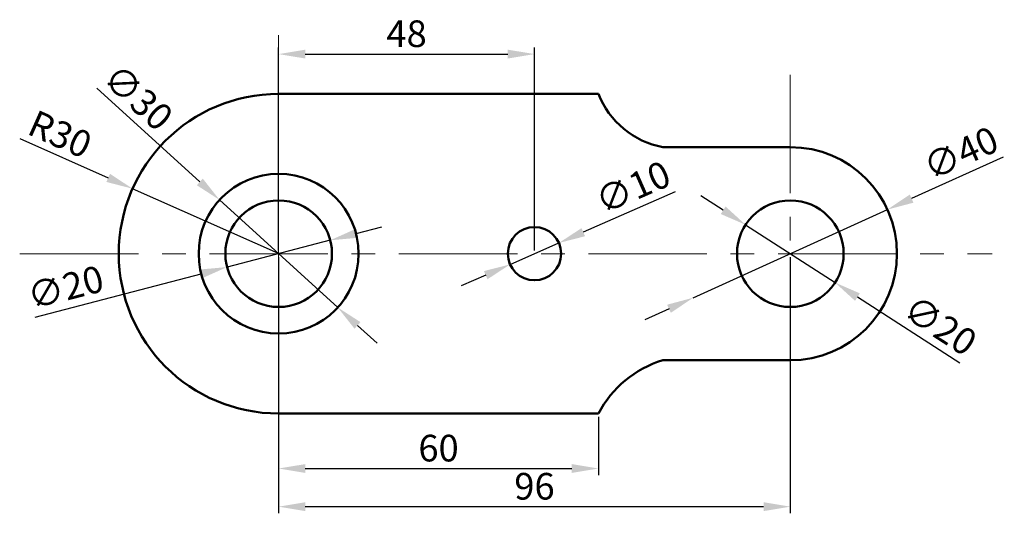
# Model space of a CAD drawing. Units: millimetres. Extents: x 1950 to 2135, y 1566 to 1659.
import ezdxf

# ---------------------------------------------------------------- set-up
doc = ezdxf.new("R2010")
doc.units = ezdxf.units.MM
doc.linetypes.add('CENTER', pattern=[50.8, 31.75, -6.35, 6.35, -6.35])
for name, color, linetype, lineweight in [('M-CNTR', 4, 'CENTER', 18), ('M-DIMS', 2, 'Continuous', 25), ('M-OUTL', 7, 'Continuous', 50)]:
    doc.layers.add(name, color=color, linetype=linetype, lineweight=lineweight)
doc.styles.get("Standard").update_dxf_attribs({"font": 'arial.ttf'})
doc.dimstyles.new('ISO-25', dxfattribs={"dimtxt": 5, "dimasz": 5, "dimexe": 1.25, "dimexo": 0.625, "dimtad": 1, "dimtxsty": 'Standard', "dimcen": 2.5, "dimadec": 0, "dimazin": 0, "dimtfac": 1, "dimtmove": 0, "dimatfit": 3, "dimfxl": 1, "dimarcsym": 0})

# ---------------------------------------------------------------- blocks, each defined once
blk = doc.blocks.new('*D1')
at = {"layer": 'Defpoints', "color": 0, "transparency": 16777216}
for p in [(2046.52, 1652.69), (1998.52, 1615.23), (2046.52, 1615.23)]:
    blk.add_point(p, dxfattribs=at)
at = {"layer": 'M-DIMS', "color": 0, "lineweight": -2, "transparency": 16777216}
for p, q in [((1998.52, 1615.85), (1998.52, 1653.94)), ((2046.52, 1615.85), (2046.52, 1653.94)), ((2003.52, 1652.69), (2041.52, 1652.69))]:
    blk.add_line(p, q, dxfattribs=at)
at = {"layer": 'M-DIMS', "color": 0, "transparency": 16777216}
for points in [[(2003.52, 1653.52), (2003.52, 1651.86), (1998.52, 1652.69)], [(2041.52, 1653.52), (2041.52, 1651.86), (2046.52, 1652.69)]]:
    blk.add_solid(points, dxfattribs=at)
at = {"layer": 'M-DIMS', "color": 0, "transparency": 16777216, "insert": (2022.52, 1655.87), "char_height": 5, "attachment_point": 5}
blk.add_mtext('48', dxfattribs=at)
blk = doc.blocks.new('*D2')
at = {"layer": 'Defpoints', "color": 0, "transparency": 16777216}
for p in [(1998.52, 1585.23), (2058.52, 1585.23), (2058.52, 1574.9)]:
    blk.add_point(p, dxfattribs=at)
at = {"layer": 'M-DIMS', "color": 0, "lineweight": -2, "transparency": 16777216}
for p, q in [((1998.52, 1584.6), (1998.52, 1573.65)), ((2058.52, 1584.6), (2058.52, 1573.65)), ((2003.52, 1574.9), (2053.52, 1574.9))]:
    blk.add_line(p, q, dxfattribs=at)
at = {"layer": 'M-DIMS', "color": 0, "transparency": 16777216}
for points in [[(2003.52, 1575.73), (2003.52, 1574.07), (1998.52, 1574.9)], [(2053.52, 1575.73), (2053.52, 1574.07), (2058.52, 1574.9)]]:
    blk.add_solid(points, dxfattribs=at)
at = {"layer": 'M-DIMS', "color": 0, "transparency": 16777216, "insert": (2028.52, 1578.08), "char_height": 5, "attachment_point": 5}
blk.add_mtext('60', dxfattribs=at)
blk = doc.blocks.new('*D3')
at = {"layer": 'Defpoints', "color": 0, "transparency": 16777216}
for p in [(1971.11, 1627.42), (1998.52, 1615.23)]:
    blk.add_point(p, dxfattribs=at)
at = {"layer": 'M-DIMS', "color": 0, "lineweight": -2, "transparency": 16777216}
for p, q in [((1949.93, 1636.85), (1966.54, 1629.46)), ((1998.52, 1615.23), (1971.11, 1627.42))]:
    blk.add_line(p, q, dxfattribs=at)
at = {"layer": 'M-DIMS', "color": 0, "transparency": 16777216}
blk.add_solid([(1966.88, 1630.22), (1966.2, 1628.69), (1971.11, 1627.42)], dxfattribs=at)
at = {"layer": 'M-DIMS', "color": 0, "transparency": 16777216, "insert": (1957.25, 1637.07), "char_height": 5, "attachment_point": 5, "rotation": 336.0117}
blk.add_mtext('R30', dxfattribs=at)
blk = doc.blocks.new('*D4')
at = {"layer": 'Defpoints', "color": 0, "transparency": 16777216}
for p in [(1987.43, 1625.32), (2009.61, 1605.13)]:
    blk.add_point(p, dxfattribs=at)
at = {"layer": 'M-DIMS', "color": 0, "lineweight": -2, "transparency": 16777216}
for p, q in [((1964.38, 1646.3), (1983.73, 1628.69)), ((2009.61, 1605.13), (1987.43, 1625.32)), ((2013.31, 1601.76), (2017.01, 1598.4))]:
    blk.add_line(p, q, dxfattribs=at)
at = {"layer": 'M-DIMS', "color": 0, "transparency": 16777216}
for points in [[(1984.29, 1629.31), (1983.17, 1628.07), (1987.43, 1625.32)], [(2013.87, 1602.38), (2012.75, 1601.15), (2009.61, 1605.13)]]:
    blk.add_solid(points, dxfattribs=at)
at = {"layer": 'M-DIMS', "color": 0, "transparency": 16777216, "insert": (1971.73, 1644.1), "char_height": 5, "attachment_point": 5, "rotation": 317.6915}
blk.add_mtext('∅30', dxfattribs=at)
blk = doc.blocks.new('*D5')
at = {"layer": 'Defpoints', "color": 0, "transparency": 16777216}
for p in [(2008.2, 1617.74), (1988.84, 1612.71)]:
    blk.add_point(p, dxfattribs=at)
at = {"layer": 'M-DIMS', "color": 0, "lineweight": -2, "transparency": 16777216}
for p, q in [((2013.04, 1619), (2017.88, 1620.26)), ((2008.2, 1617.74), (1988.84, 1612.71)), ((1952.82, 1603.34), (1984, 1611.45))]:
    blk.add_line(p, q, dxfattribs=at)
at = {"layer": 'M-DIMS', "color": 0, "transparency": 16777216}
for points in [[(2012.83, 1619.81), (2013.25, 1618.2), (2008.2, 1617.74)], [(1983.79, 1612.26), (1984.21, 1610.64), (1988.84, 1612.71)]]:
    blk.add_solid(points, dxfattribs=at)
at = {"layer": 'M-DIMS', "color": 0, "transparency": 16777216, "insert": (1958.68, 1608.29), "char_height": 5, "attachment_point": 5, "rotation": 14.5827}
blk.add_mtext('∅20', dxfattribs=at)
blk = doc.blocks.new('*D6')
at = {"layer": 'Defpoints', "color": 0, "transparency": 16777216}
for p in [(2086.12, 1620.66), (2102.92, 1609.8)]:
    blk.add_point(p, dxfattribs=at)
at = {"layer": 'M-DIMS', "color": 0, "lineweight": -2, "transparency": 16777216}
for p, q in [((2081.92, 1623.37), (2077.73, 1626.09)), ((2086.12, 1620.66), (2102.92, 1609.8)), ((2126.31, 1594.67), (2107.12, 1607.08))]:
    blk.add_line(p, q, dxfattribs=at)
at = {"layer": 'M-DIMS', "color": 0, "transparency": 16777216}
for points in [[(2082.38, 1624.07), (2081.47, 1622.67), (2086.12, 1620.66)], [(2107.57, 1607.78), (2106.66, 1606.38), (2102.92, 1609.8)]]:
    blk.add_solid(points, dxfattribs=at)
at = {"layer": 'M-DIMS', "color": 0, "transparency": 16777216, "insert": (2122.3, 1601.22), "char_height": 5, "attachment_point": 5, "rotation": 327.1147}
blk.add_mtext('∅20', dxfattribs=at)
blk = doc.blocks.new('*D7')
at = {"layer": 'Defpoints', "color": 0, "transparency": 16777216}
for p in [(2112.73, 1623.5), (2076.31, 1606.96)]:
    blk.add_point(p, dxfattribs=at)
at = {"layer": 'M-DIMS', "color": 0, "lineweight": -2, "transparency": 16777216}
for p, q in [((2134.43, 1633.35), (2117.28, 1625.56)), ((2076.31, 1606.96), (2112.73, 1623.5)), ((2071.76, 1604.89), (2067.21, 1602.82))]:
    blk.add_line(p, q, dxfattribs=at)
at = {"layer": 'M-DIMS', "color": 0, "transparency": 16777216}
for points in [[(2116.94, 1626.32), (2117.63, 1624.8), (2112.73, 1623.5)], [(2071.41, 1605.65), (2072.1, 1604.13), (2076.31, 1606.96)]]:
    blk.add_solid(points, dxfattribs=at)
at = {"layer": 'M-DIMS', "color": 0, "transparency": 16777216, "insert": (2126.76, 1633.51), "char_height": 5, "attachment_point": 5, "rotation": 24.423}
blk.add_mtext('∅40', dxfattribs=at)
blk = doc.blocks.new('*D8')
at = {"layer": 'Defpoints', "color": 0, "transparency": 16777216}
for p in [(1998.52, 1615.23), (2094.52, 1615.23), (2094.52, 1567.74)]:
    blk.add_point(p, dxfattribs=at)
at = {"layer": 'M-DIMS', "color": 0, "lineweight": -2, "transparency": 16777216}
for p, q in [((1998.52, 1614.6), (1998.52, 1566.49)), ((2094.52, 1614.6), (2094.52, 1566.49)), ((2003.52, 1567.74), (2089.52, 1567.74))]:
    blk.add_line(p, q, dxfattribs=at)
at = {"layer": 'M-DIMS', "color": 0, "transparency": 16777216}
for points in [[(2003.52, 1568.57), (2003.52, 1566.91), (1998.52, 1567.74)], [(2089.52, 1568.57), (2089.52, 1566.91), (2094.52, 1567.74)]]:
    blk.add_solid(points, dxfattribs=at)
at = {"layer": 'M-DIMS', "color": 0, "transparency": 16777216, "insert": (2046.52, 1570.92), "char_height": 5, "attachment_point": 5}
blk.add_mtext('96', dxfattribs=at)
blk = doc.blocks.new('*D9')
at = {"layer": 'Defpoints', "color": 0, "transparency": 16777216}
for p in [(2051.1, 1617.24), (2041.94, 1613.21)]:
    blk.add_point(p, dxfattribs=at)
at = {"layer": 'M-DIMS', "color": 0, "lineweight": -2, "transparency": 16777216}
for p, q in [((2072.91, 1626.85), (2055.67, 1619.26)), ((2041.94, 1613.21), (2051.1, 1617.24)), ((2037.37, 1611.2), (2032.79, 1609.18))]:
    blk.add_line(p, q, dxfattribs=at)
at = {"layer": 'M-DIMS', "color": 0, "transparency": 16777216}
for points in [[(2055.34, 1620.02), (2056.01, 1618.5), (2051.1, 1617.24)], [(2037.03, 1611.96), (2037.71, 1610.43), (2041.94, 1613.21)]]:
    blk.add_solid(points, dxfattribs=at)
at = {"layer": 'M-DIMS', "color": 0, "transparency": 16777216, "insert": (2065.24, 1627.1), "char_height": 5, "attachment_point": 5, "rotation": 23.7744}
blk.add_mtext('∅10', dxfattribs=at)

msp = doc.modelspace()

# ---------------------------------------------------------------- linework, layer by layer
at = {"layer": 'M-CNTR', "ltscale": 0.7}
for p, q in [((1998.521, 1656.212), (1998.521, 1575.334)), ((2094.521, 1648.792), (2094.521, 1584.733)), ((1949.972, 1615.227), (2132.407, 1615.227))]:
    msp.add_line(p, q, dxfattribs=at)
at = {"layer": 'M-OUTL'}
for p, q in [((1998.521, 1645.227), (2058.521, 1645.227)), ((2094.521, 1635.227), (2070.597, 1635.227)), ((2094.521, 1595.227), (2070.597, 1595.227)), ((1998.521, 1585.227), (2058.521, 1585.227))]:
    msp.add_line(p, q, dxfattribs=at)
for centre, radius in [((1998.521, 1615.227), 15), ((1998.521, 1615.227), 10), ((2094.521, 1615.227), 10), ((2046.521, 1615.227), 5)]:
    msp.add_circle(centre, radius, dxfattribs=at)
for centre, radius, start, end in [((1998.521, 1615.227), 30, 90, 270), ((2073.643, 1651.197), 16.258, 201.5446, 259.20298), ((2094.521, 1615.227), 20, 270, 90), ((2076.578, 1575.712), 20.411, 107.03879, 152.21363)]:
    msp.add_arc(centre, radius, start, end, dxfattribs=at)

# ---------------------------------------------------------------- dimensions: what is measured, and where the dimension line sits
at = {"layer": 'M-DIMS'}
for base, p1, p2, picture, middle in [((2046.521, 1652.69), (1998.521, 1615.227), (2046.521, 1615.227), '*D1', (2022.521, 1655.868)), ((2094.521, 1567.741), (1998.521, 1615.227), (2094.521, 1615.227), '*D8', (2046.521, 1570.919)), ((2058.521, 1574.901), (1998.521, 1585.227), (2058.521, 1585.227), '*D2', (2028.521, 1578.079))]:
    dim = msp.add_linear_dim(base=base, p1=p1, p2=p2, dimstyle='ISO-25', override={"dimclrd": 0, "dimclre": 0, "dimclrt": 0}, dxfattribs=at)
    dim.commit()
    dim.dimension.update_dxf_attribs({"geometry": picture, "text_midpoint": middle})
for p1, p2, picture, middle in [((2009.614, 1605.13), (1987.428, 1625.324), '*D4', (1969.493, 1641.648)), ((2086.123, 1620.657), (2102.918, 1609.797), '*D6', (2120.501, 1598.429)), ((2008.198, 1617.745), (1988.843, 1612.709), '*D5', (1959.511, 1605.078))]:
    dim = msp.add_diameter_dim_2p(p1=p1, p2=p2, dimstyle='ISO-25', override={"dimclrd": 0, "dimclre": 0, "dimclrt": 0}, dxfattribs=at)
    dim.commit()
    dim.dimension.update_dxf_attribs({"geometry": picture, "text_midpoint": middle, "dimtype": 163})
dim = msp.add_radius_dim(center=(1998.521, 1615.227), mpoint=(1971.112, 1627.423), dimstyle='ISO-25', override={"dimclrd": 0, "dimclre": 0, "dimclrt": 0}, dxfattribs=at)
dim.commit()
dim.dimension.update_dxf_attribs({"geometry": '*D3', "text_midpoint": (1957.247, 1637.073)})
for p1, p2, picture, middle in [((2076.31, 1606.958), (2112.731, 1623.496), '*D7', (2126.763, 1633.512)), ((2041.945, 1613.211), (2051.096, 1617.243), '*D9', (2065.241, 1627.099))]:
    dim = msp.add_diameter_dim_2p(p1=p1, p2=p2, dimstyle='ISO-25', override={"dimclrd": 0, "dimclre": 0, "dimclrt": 0}, dxfattribs=at)
    dim.commit()
    dim.dimension.update_dxf_attribs({"geometry": picture, "text_midpoint": middle})

doc.saveas('drawing.dxf')
